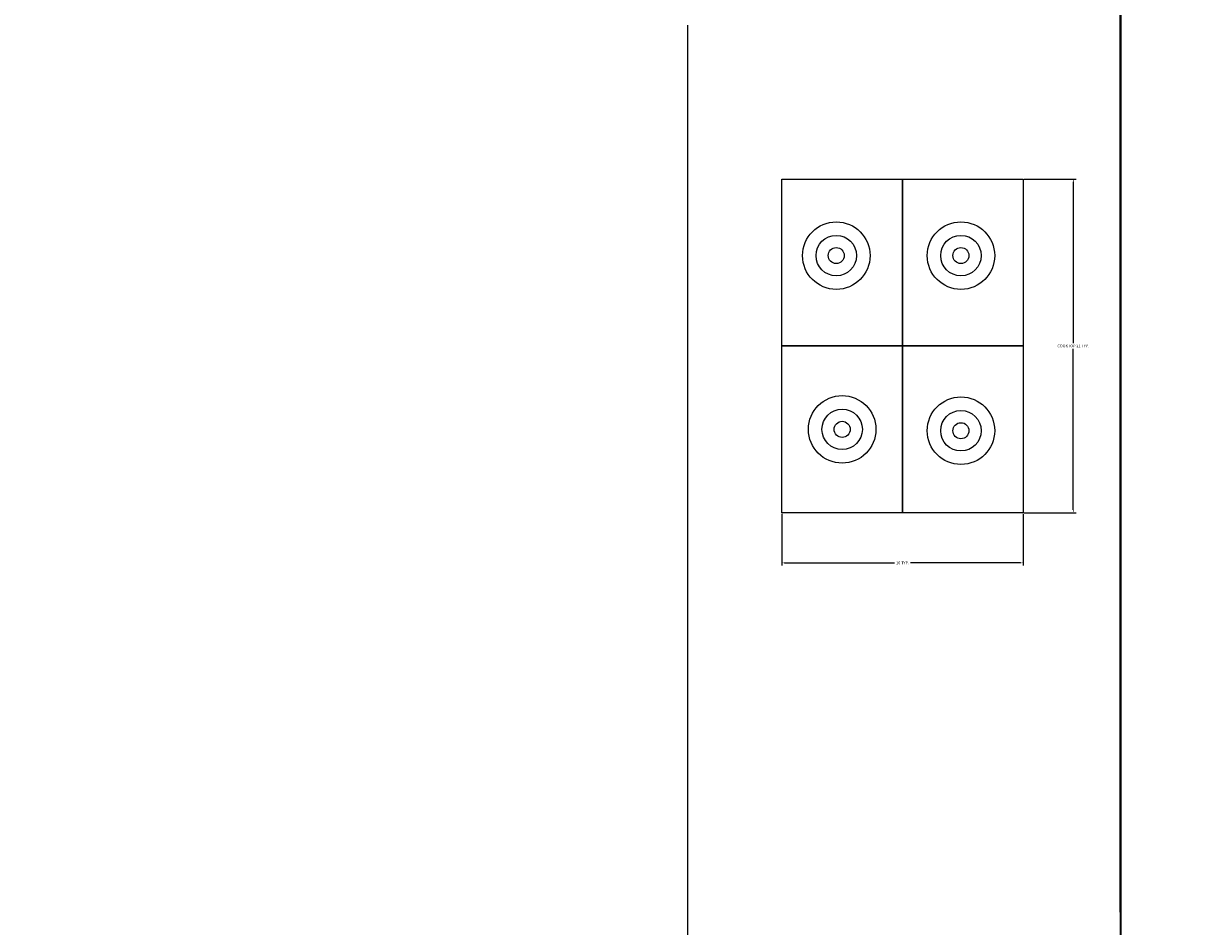
# Model space of a CAD drawing. Units: millimetres. Extents: x 27017497 to 27018854, y 7058029 to 7059154.
# Tile 51 of 91: x 27017962 to 27018038, y 7058236 to 7058294. Entities that reach past the tile are written whole.
import ezdxf

# ---------------------------------------------------------------- set-up
doc = ezdxf.new("R2010")
doc.units = ezdxf.units.MM
for name, color, linetype, lineweight in [('A-ANNO-DIMS', 2, 'Continuous', 18), ('A-EQPM', 9, 'Continuous', 18), ('A-FLOR-CASE', 8, 'Continuous', 20), ('A-WALL', 7, 'Continuous', 35)]:
    doc.layers.add(name, color=color, linetype=linetype, lineweight=lineweight)
doc.styles.get("Standard").update_dxf_attribs({"font": 'arial.ttf'})
doc.dimstyles.get("Standard").update_dxf_attribs({"dimtxt": 0.18, "dimasz": 0.18, "dimexe": 0.18, "dimexo": 0.0625, "dimgap": 0.09, "dimtad": 0, "dimtih": 1, "dimtoh": 1, "dimdec": 4, "dimzin": 0, "dimdsep": 46, "dimtxsty": 'Standard', "dimcen": 0.09, "dimadec": 0, "dimazin": 0, "dimtfac": 1, "dimtdec": 4, "dimtofl": 0, "dimtmove": 0, "dimatfit": 3, "dimfxl": 1, "dimtolj": 1, "dimtzin": 0, "dimarcsym": 0})

# ---------------------------------------------------------------- blocks, each defined once
blk = doc.blocks.new('COOKTOP-FOUR-BURNER')
for points in [[(7.753, 21.43), (7.753, 10.715), (0, 10.715), (0, 21.43)], [(15.506, 21.43), (15.506, 10.715), (7.753, 10.715), (7.753, 21.43)], [(7.753, 10.715), (7.753, 0), (0, 0), (0, 10.715)], [(15.506, 10.715), (15.506, 0), (7.753, 0), (7.753, 10.715)]]:
    blk.add_lwpolyline(points, close=True)
for centre, radius in [((3.498, 16.514), 2.167), ((11.503, 16.514), 2.167), ((3.498, 16.514), 1.298), ((11.503, 16.514), 1.298), ((3.498, 16.514), 0.515), ((3.498, 16.514), 0.515), ((11.503, 16.514), 0.515), ((11.503, 16.514), 0.515), ((3.876, 5.358), 2.167), ((11.503, 5.271), 2.167), ((3.876, 5.358), 1.298), ((11.503, 5.271), 1.298), ((3.876, 5.358), 0.515), ((3.876, 5.358), 0.515), ((11.503, 5.271), 0.515), ((11.503, 5.271), 0.515)]:
    blk.add_circle(centre, radius)
blk = doc.blocks.new('*D43')
at = {"layer": 'A-ANNO-DIMS', "color": 0, "lineweight": -2, "transparency": 16777216}
for p, q in [((27018025.995, 7058284.433), (27018029.327, 7058284.433)), ((27018029.147, 7058284.253), (27018029.147, 7058273.901)), ((27018029.147, 7058263.183), (27018029.147, 7058273.535)), ((27018025.995, 7058263.003), (27018029.327, 7058263.003))]:
    blk.add_line(p, q, dxfattribs=at)
at = {"layer": 'A-ANNO-DIMS', "color": 0, "transparency": 16777216}
for points in [[(27018029.117, 7058284.253), (27018029.177, 7058284.253), (27018029.147, 7058284.433)], [(27018029.117, 7058263.183), (27018029.177, 7058263.183), (27018029.147, 7058263.003)]]:
    blk.add_solid(points, dxfattribs=at)
at = {"layer": 'Defpoints', "color": 0, "transparency": 16777216}
for p in [(27018025.933, 7058284.433), (27018029.147, 7058284.433), (27018025.933, 7058263.003)]:
    blk.add_point(p, dxfattribs=at)
at = {"layer": 'A-ANNO-DIMS', "color": 0, "transparency": 16777216, "insert": (27018029.147, 7058273.718), "char_height": 0.18, "attachment_point": 5}
blk.add_mtext('\\A1;COOKTOP 21 TYP.', dxfattribs=at)
blk = doc.blocks.new('*D44')
at = {"layer": 'A-ANNO-DIMS', "color": 0, "lineweight": -2, "transparency": 16777216}
for p, q in [((27018010.427, 7058262.941), (27018010.427, 7058259.609)), ((27018025.933, 7058262.941), (27018025.933, 7058259.609)), ((27018010.607, 7058259.789), (27018017.66, 7058259.789)), ((27018025.753, 7058259.789), (27018018.699, 7058259.789))]:
    blk.add_line(p, q, dxfattribs=at)
at = {"layer": 'A-ANNO-DIMS', "color": 0, "transparency": 16777216}
for points in [[(27018010.607, 7058259.819), (27018010.607, 7058259.759), (27018010.427, 7058259.789)], [(27018025.753, 7058259.819), (27018025.753, 7058259.759), (27018025.933, 7058259.789)]]:
    blk.add_solid(points, dxfattribs=at)
at = {"layer": 'Defpoints', "color": 0, "transparency": 16777216}
for p in [(27018010.427, 7058263.003), (27018025.933, 7058263.003), (27018025.933, 7058259.789)]:
    blk.add_point(p, dxfattribs=at)
at = {"layer": 'A-ANNO-DIMS', "color": 0, "transparency": 16777216, "insert": (27018018.18, 7058259.789), "char_height": 0.18, "attachment_point": 5}
blk.add_mtext('\\A1;16 TYP.', dxfattribs=at)
blk = doc.blocks.new('*D47')
at = {"layer": 'A-ANNO-DIMS', "color": 0, "lineweight": -2, "transparency": 16777216}
for p, q in [((27017561.166, 7058294.35), (27017561.166, 7058028.6)), ((27018790.606, 7058294.35), (27018790.606, 7058028.6)), ((27017561.346, 7058028.78), (27018175.431, 7058028.78)), ((27018790.426, 7058028.78), (27018176.341, 7058028.78))]:
    blk.add_line(p, q, dxfattribs=at)
at = {"layer": 'A-ANNO-DIMS', "color": 0, "transparency": 16777216}
for points in [[(27017561.346, 7058028.81), (27017561.346, 7058028.75), (27017561.166, 7058028.78)], [(27018790.426, 7058028.81), (27018790.426, 7058028.75), (27018790.606, 7058028.78)]]:
    blk.add_solid(points, dxfattribs=at)
at = {"layer": 'Defpoints', "color": 0, "transparency": 16777216}
for p in [(27017561.166, 7058294.412), (27018790.606, 7058294.412), (27018790.606, 7058028.78)]:
    blk.add_point(p, dxfattribs=at)
at = {"layer": 'A-ANNO-DIMS', "color": 0, "transparency": 16777216, "insert": (27018175.886, 7058028.78), "char_height": 0.18, "attachment_point": 5}
blk.add_mtext('\\A1;1229.4', dxfattribs=at)
blk = doc.blocks.new('*D48')
at = {"layer": 'A-ANNO-DIMS', "color": 0, "lineweight": -2, "transparency": 16777216}
for p, q in [((27018463.498, 7058622.912), (27017497.536, 7058622.912)), ((27017497.716, 7058622.732), (27017497.716, 7058357.753)), ((27017497.716, 7058092.41), (27017497.716, 7058357.389)), ((27018555.129, 7058092.23), (27017497.536, 7058092.23))]:
    blk.add_line(p, q, dxfattribs=at)
at = {"layer": 'A-ANNO-DIMS', "color": 0, "transparency": 16777216}
for points in [[(27017497.686, 7058622.732), (27017497.746, 7058622.732), (27017497.716, 7058622.912)], [(27017497.686, 7058092.41), (27017497.746, 7058092.41), (27017497.716, 7058092.23)]]:
    blk.add_solid(points, dxfattribs=at)
at = {"layer": 'Defpoints', "color": 0, "transparency": 16777216}
for p in [(27018463.561, 7058622.912), (27017497.716, 7058092.23), (27018555.192, 7058092.23)]:
    blk.add_point(p, dxfattribs=at)
at = {"layer": 'A-ANNO-DIMS', "color": 0, "transparency": 16777216, "insert": (27017497.716, 7058357.571), "char_height": 0.18, "attachment_point": 5}
blk.add_mtext('\\A1;530.7', dxfattribs=at)

msp = doc.modelspace()

# ---------------------------------------------------------------- linework, layer by layer
at = {"layer": 'A-FLOR-CASE'}
msp.add_line((27018004.365, 7058294.322), (27018004.365, 7058223.172), dxfattribs=at)
at = {"layer": 'A-WALL'}
msp.add_line((27018032.166, 7058386.803), (27018032.166, 7058141.912), dxfattribs=at)
msp.add_lwpolyline([(27018032.178, 7058237.363), (27018032.178, 7058375.363)], dxfattribs=at)

# ---------------------------------------------------------------- block references
at = {"layer": 'A-EQPM'}
msp.add_blockref('COOKTOP-FOUR-BURNER', (27018010.427, 7058263.003), dxfattribs=at)

# ---------------------------------------------------------------- dimensions: what is measured, and where the dimension line sits
at = {"layer": 'A-ANNO-DIMS'}
dim = msp.add_linear_dim(base=(27017497.716, 7058092.23), p1=(27018463.561, 7058622.912), p2=(27018555.192, 7058092.23), angle=90, dimstyle='Standard', override={"dimdec": 1, "dimlfac": 1, "dimrnd": 0, "dimzin": 0, "dimdsep": 46, "dimlunit": 2}, dxfattribs=at)
dim.commit()
dim.dimension.update_dxf_attribs({"geometry": '*D48', "text_midpoint": (27017497.716, 7058357.571)})
dim = msp.add_linear_dim(base=(27018790.606, 7058028.78), p1=(27017561.166, 7058294.412), p2=(27018790.606, 7058294.412), dimstyle='Standard', override={"dimdec": 1, "dimlfac": 1, "dimrnd": 0, "dimzin": 0, "dimdsep": 46, "dimlunit": 2}, dxfattribs=at)
dim.commit()
dim.dimension.update_dxf_attribs({"geometry": '*D47', "text_midpoint": (27018175.886, 7058028.78)})
dim = msp.add_linear_dim(base=(27018029.147, 7058284.433), p1=(27018025.933, 7058263.003), p2=(27018025.933, 7058284.433), angle=90, text='COOKTOP <> TYP.', dimstyle='Standard', override={"dimdec": 0, "dimlfac": 1, "dimrnd": 0, "dimzin": 0, "dimdsep": 46, "dimlunit": 2}, dxfattribs=at)
dim.commit()
dim.dimension.update_dxf_attribs({"geometry": '*D43', "text_midpoint": (27018029.147, 7058273.718)})
dim = msp.add_linear_dim(base=(27018025.933, 7058259.789), p1=(27018010.427, 7058263.003), p2=(27018025.933, 7058263.003), text='<> TYP.', dimstyle='Standard', override={"dimdec": 0, "dimlfac": 1, "dimrnd": 0, "dimzin": 0, "dimdsep": 46, "dimlunit": 2}, dxfattribs=at)
dim.commit()
dim.dimension.update_dxf_attribs({"geometry": '*D44', "text_midpoint": (27018018.18, 7058259.789)})

doc.saveas('drawing.dxf')
